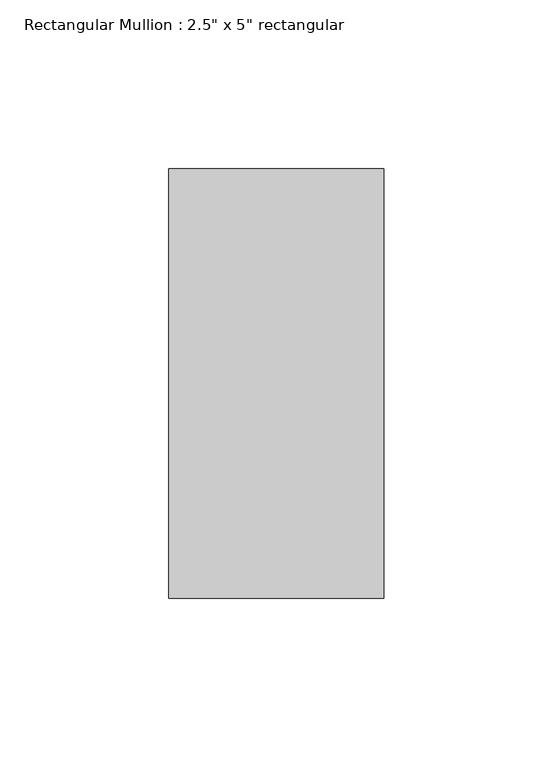
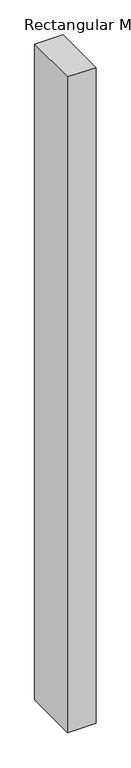
"""IFC4 building model written with IfcOpenShell, lengths in millimetres: member geometry."""

from ifc_helpers import new_model, si_unit, frame, origin, place, context, project, spatial, polyline, outline, extrude, source, transform, mapped, element, save


def member_3e567bd2(model_context):
    return source(origin(), model_context, "Body", "SweptSolid", [
        extrude(outline(polyline([(0.0, 63.5), (0.0, -63.5), (-63.5, -63.5), (-63.5, 63.5), (0.0, 63.5)])), frame((0.0, 0.0, -1550.2845828), z_axis=(0.0, 0.0, 1.0), x_axis=(1.0, 0.0, 0.0)), (0.0, 0.0, 1.0), 1550.2845828),
    ])


if __name__ == "__main__":
    model = new_model("IFC4")
    model_context = context("Model", 3, world=origin())
    ifc_project = project(units=[si_unit("LENGTHUNIT", "METRE", prefix="MILLI")], contexts=[model_context])
    site = spatial("IfcSite", under=ifc_project)
    building = spatial("IfcBuilding", under=site)
    placement = place(None, origin())
    member_shape = member_3e567bd2(model_context)
    element("IfcMember", 1, ObjectType="Rectangular Mullion : 2.5\" x 5\" rectangular", at=placement, inside=building, context=model_context, shape_type="MappedRepresentation", body=[
        mapped(member_shape, transform((0.0, 0.0, 0.0), x_axis=(1.0, 0.0, 0.0), y_axis=(0.0, 1.0, 0.0), z_axis=(0.0, 0.0, 1.0))),
    ])
    save(model, "model.ifc")

# Revit data of these elements
# Type "Rectangular Mullion : 2.5\" x 5\" rectangular"
#   built-in parameter 1007304 = 0.416667 (stored number, unit not read)
#   built-in parameter 1007301 = 0.104167 (stored number, unit not read)
#   built-in parameter 1007300 = 0.104167 (stored number, unit not read)
# Element 1 (IfcMember, "Rectangular Mullion : 2.5\" x 5\" rectangular")
#   Materials on its faces: "Aluminum"
# Materials
#   "Aluminum": class "Metal", colour RGB 247 247 247, transparency 0, Description = "Aluminum 6061", Cost = 0
